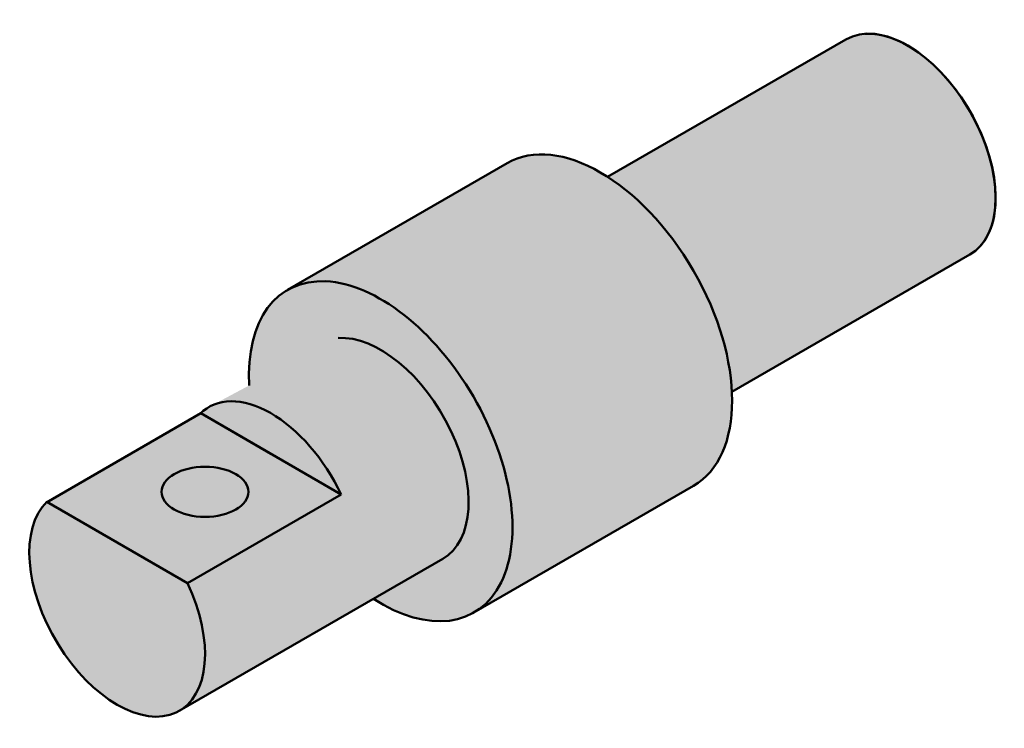
# Model space of a CAD drawing. Units: inches. Extents: x 105 to 6825, y 111 to 6061.
# Tile 1 of 2: x 105 to 299, y 111 to 250. Entities that reach past the tile are written whole.
import ezdxf

# ---------------------------------------------------------------- set-up
doc = ezdxf.new("R2010")
doc.units = ezdxf.units.IN
doc.header["$MEASUREMENT"] = 0
doc.layers.add('M-HATC', color=8, linetype='Continuous', lineweight=18)
doc.layers.add('M-OUTL', color=7, linetype='Continuous', lineweight=50)

msp = doc.modelspace()

# ---------------------------------------------------------------- hatches: boundary and pattern name
at = {"layer": 'M-HATC'}
h = msp.add_hatch(color=256, dxfattribs=at)
h.dxf.hatch_style = 1
h.set_gradient(color1=(99, 100, 102), tint=1, name='INVCYLINDER')
edge = h.paths.add_edge_path()
edge.add_ellipse((219.2829557775919, 190.3354462005651), major_axis=(18.37117307087383, -31.81980515339464), ratio=0.577350269189626, start_angle=392.8421304144117, end_angle=507.1578695855882)
edge.add_ellipse((219.2829557775919, 190.3354462005651), major_axis=(18.37117307087383, -31.81980515339464), ratio=0.577350269189626, start_angle=507.1578695855882, end_angle=540)
edge.add_line((200.9117827067181, 222.1552513539597), (157.6105125174961, 197.1552513539597))
edge.add_ellipse((175.9816855883699, 165.3354462005651), major_axis=(18.37117307087383, -31.81980515339464), ratio=0.577350269189626, start_angle=359.99999999999994, end_angle=540, ccw=False)
edge.add_line((194.3528586592437, 133.5156410471704), (237.6541288484657, 158.5156410471704))
edge.add_ellipse((219.2829557775919, 190.3354462005651), major_axis=(18.37117307087383, -31.81980515339464), ratio=0.577350269189626, start_angle=360, end_angle=392.8421304144117)
edge = h.paths.add_edge_path(flags=16)
edge.add_ellipse((197.6323206829809, 207.8354462005651), major_axis=(-8.573214099741122, 0), ratio=0.5773502691896255, start_angle=0, end_angle=360)
edge = h.paths.add_edge_path()
edge.add_ellipse((279.9047340425026, 225.3354462005651), major_axis=(12.24744871391588, -21.21320343559644), ratio=0.5773502691896262, start_angle=360, end_angle=530.6170018609903)
edge.add_ellipse((279.9047340425026, 225.3354462005651), major_axis=(12.24744871391588, -21.21320343559644), ratio=0.5773502691896262, start_angle=530.6170018609903, end_angle=540)
edge.add_line((267.6572853285871, 246.5486496361617), (220.7285710013052, 219.4543437865824))
edge.add_ellipse((219.2829557775919, 190.3354462005651), major_axis=(18.37117307087383, -31.81980515339464), ratio=0.577350269189626, start_angle=392.8421304144117, end_angle=507.1578695855882, ccw=False)
edge.add_line((245.223468429137, 177.0279369153896), (292.1521827564183, 204.1222427649685))
edge = h.paths.add_edge_path(flags=16)
edge.add_ellipse((243.8023449814453, 215.4109931062057), major_axis=(-6.123724356957945, 0), ratio=0.577350269189626, start_angle=388.5479502745485, end_angle=509.9999999999999, ccw=False)
edge.add_ellipse((243.8023449814453, 215.4109931062057), major_axis=(-6.123724356957945, 0), ratio=0.577350269189626, start_angle=329.99999999999994, end_angle=388.5479502745485, ccw=False)
edge.add_line((239.4722179625231, 217.9109931062057), (270.6491324987629, 235.9109931062057))
edge.add_ellipse((274.9792595176852, 233.4109931062057), major_axis=(-6.123724356957945, 0), ratio=0.577350269189626, start_angle=150, end_angle=329.99999999999994, ccw=False)
edge.add_line((279.3093865366074, 230.9109931062057), (248.1324720003676, 212.9109931062057))
edge = h.paths.add_edge_path()
edge.add_ellipse((175.9816855883699, 165.3354462005651), major_axis=(12.24744871391589, -21.21320343559642), ratio=0.577350269189626, start_angle=360, end_angle=530.6170018609903)
edge.add_line((167.577058087087, 187.6754647729887), (142.3182689200914, 174.1790395580179))
edge.add_ellipse((154.331050493759, 152.8354462005651), major_axis=(12.24744871391589, -21.21320343559642), ratio=0.5773502691896258, start_angle=436.10211375198594, end_angle=539.3720471364466, ccw=False)
edge.add_line((168.18745695431, 156.8354462005651), (137.8765678218547, 139.3354462005651))
edge.add_ellipse((124.0201613613036, 135.3354462005651), major_axis=(12.24744871391589, -21.21320343559642), ratio=0.577350269189626, start_angle=359.99999999999994, end_angle=436.102113751986, ccw=False)
edge.add_line((136.2676100752195, 114.1222427649686), (188.2291343022859, 144.1222427649687))
edge = h.paths.add_edge_path()
edge.add_ellipse((124.0201613613036, 135.3354462005651), major_axis=(12.24744871391589, -21.21320343559642), ratio=0.577350269189626, start_angle=360, end_angle=436.1021137519859)
edge.add_line((137.8765678218547, 139.335446200565), (124.0201613613036, 147.3354462005651))
edge.add_line((124.0201613613036, 147.3354462005651), (110.1997146436663, 155.3146848333139))
edge.add_line((110.1997146436663, 155.3146848333139), (110.0602307690168, 155.2341537807374))
edge.add_ellipse((124.0201613613036, 135.3354462005651), major_axis=(12.24744871391589, -21.21320343559642), ratio=0.577350269189626, start_angle=185.0515649198831, end_angle=360)
h = msp.add_hatch(color=256, dxfattribs=at)
h.dxf.hatch_style = 1
h.set_gradient(color1=(205, 105, 40), color2=(254, 204, 102), tint=1, name='INVCYLINDER')
edge = h.paths.add_edge_path()
edge.add_ellipse((175.9816855883699, 165.3354462005651), major_axis=(18.37117307087383, -31.81980515339464), ratio=0.577350269189626, start_angle=360, end_angle=540)
edge.add_ellipse((175.9816855883699, 165.3354462005651), major_axis=(18.37117307087383, -31.81980515339464), ratio=0.577350269189626, start_angle=540, end_angle=213.4043430439043)
edge.add_line((150.0580240784876, 178.3145911866752), (167.577058087087, 187.6754647729887))
edge.add_ellipse((175.9816855883699, 165.3354462005651), major_axis=(12.24744871391589, -21.21320343559642), ratio=0.577350269189626, start_angle=360, end_angle=530.6170018609904, ccw=False)
edge.add_line((188.2291343022859, 144.1222427649687), (174.5360703646567, 136.2165486145477))
edge.add_ellipse((175.9816855883699, 165.3354462005651), major_axis=(18.37117307087383, -31.81980515339464), ratio=0.577350269189626, start_angle=327.1578695855883, end_angle=360)
edge = h.paths.add_edge_path()
edge.add_ellipse((154.331050493759, 152.8354462005651), major_axis=(12.24744871391589, -21.21320343559642), ratio=0.5773502691896258, start_angle=436.1021137519858, end_angle=539.3720471364466)
edge.add_ellipse((154.331050493759, 152.8354462005651), major_axis=(12.24744871391589, -21.21320343559642), ratio=0.5773502691896258, start_angle=539.3720471364466, end_angle=185.0515649198831)
edge.add_line((140.4830409542333, 172.8305982359507), (168.18745695431, 156.8354462005651))
edge = h.paths.add_edge_path()
edge.add_ellipse((274.7326623839076, 228.4170778232225), major_axis=(-6.123724356957945, 0), ratio=0.577350269189626, start_angle=208.5479502745484, end_angle=329.99999999999994, ccw=False)
edge.add_line((279.1894483769248, 230.8417467774269), (279.3093865366074, 230.9109931062057))
edge.add_ellipse((274.9792595176852, 233.4109931062057), major_axis=(-6.123724356957945, 0), ratio=0.577350269189626, start_angle=149.9999999999999, end_angle=329.9999999999999)
edge.add_line((270.6491324987628, 235.9109931062056), (239.4722179625231, 217.9109931062057))
edge.add_ellipse((243.8023449814453, 215.4109931062057), major_axis=(-6.123724356957945, 0), ratio=0.577350269189626, start_angle=329.9999999999999, end_angle=388.5479502745485)
edge.add_line((239.3455589884283, 212.9863241520014), (270.4025353649857, 230.9170778232227))
h = msp.add_hatch(color=256, dxfattribs=at)
h.dxf.hatch_style = 1
h.set_gradient(color1=(205, 105, 40), color2=(254, 204, 102), tint=1, name='INVCYLINDER')
h.paths.add_polyline_path([(168.18745695431, 156.8354462005651), (140.5106037761216, 172.8146848333139), (110.1997146436663, 155.3146848333139), (124.0201613613036, 147.3354462005651), (137.8765678218547, 139.3354462005651)])
edge = h.paths.add_edge_path(flags=16)
edge.add_ellipse((141.3406694369924, 157.3354462005651), major_axis=(-8.573214099741122, 0), ratio=0.5773502691896255, start_angle=0, end_angle=360)
edge = h.paths.add_edge_path()
edge.add_ellipse((197.6323206829809, 207.8354462005651), major_axis=(-8.573214099741122, 0), ratio=0.5773502691896255, start_angle=0, end_angle=360)
edge = h.paths.add_edge_path()
edge.add_ellipse((274.7326623839076, 228.4170778232225), major_axis=(-6.123724356957945, 0), ratio=0.577350269189626, start_angle=208.5479502745484, end_angle=329.9999999999999)
edge.add_line((270.4025353649857, 230.9170778232227), (239.3455589884283, 212.9863241520014))
edge.add_ellipse((243.8023449814453, 215.4109931062057), major_axis=(-6.123724356957945, 0), ratio=0.577350269189626, start_angle=388.5479502745485, end_angle=509.9999999999999)
edge.add_line((248.1324720003674, 212.9109931062056), (279.1894483769248, 230.8417467774269))
h = msp.add_hatch(color=256, dxfattribs=at)
h.dxf.hatch_style = 1
h.set_gradient(color1=(153, 27, 30), color2=(254, 204, 102), tint=1, name='INVCYLINDER')
edge = h.paths.add_edge_path()
edge.add_ellipse((197.6323206829809, 207.8354462005651), major_axis=(-8.573214099741122, 0), ratio=0.5773502691896255, start_angle=0, end_angle=360)
edge = h.paths.add_edge_path()
edge.add_ellipse((141.3406694369924, 157.3354462005651), major_axis=(-8.573214099741122, 0), ratio=0.5773502691896255, start_angle=0, end_angle=360)

# ---------------------------------------------------------------- linework, layer by layer
at = {"layer": 'M-OUTL'}
for p, q in [((267.6572853285867, 246.5486496361615), (220.7285710013052, 219.4543437865824)), ((157.6105125174961, 197.1552513539597), (200.9117827067181, 222.1552513539597)), ((292.1521827564185, 204.1222427649686), (245.223468429137, 177.0279369153896)), ((110.0602307690168, 155.2341537807374), (140.5106037761216, 172.8146848333139)), ((154.331050493759, 164.8354462005651), (140.5106037761216, 172.8146848333139)), ((140.5106037761216, 172.8146848333139), (168.18745695431, 156.8354462005651)), ((194.3528586592438, 133.5156410471704), (237.6541288484657, 158.5156410471704)), ((124.0201613613036, 147.3354462005651), (110.1637549007526, 155.3354462005651)), ((137.8765678218547, 139.3354462005651), (168.18745695431, 156.8354462005651)), ((124.0201613613036, 147.3354462005651), (137.8765678218547, 139.3354462005651)), ((188.2291343022858, 144.1222427649686), (136.2676100752195, 114.1222427649686)), ((136.2676100752195, 114.1222427649686), (188.2291343022859, 144.1222427649687))]:
    msp.add_line(p, q, dxfattribs=at)
for centre, major_axis, ratio, start_param, end_param in [((279.9047340425026, 225.3354462005651), (12.24744871391588, -21.21320343559644), 0.5773502691896262, 6.283185307179586, 9.42477796076938), ((279.9047340425026, 225.335446200565), (12.24744871391589, -21.21320343559642), 0.577350269189626, 6.283185307179586, 9.146019019490385), ((219.2829557775919, 190.3354462005651), (18.37117307087383, -31.81980515339464), 0.577350269189626, 6.283185307179586, 9.42477796076938), ((175.9816855883699, 165.3354462005651), (18.37117307087383, -31.81980515339464), 0.577350269189626, 5.442116636611656, 10.27648764334619), ((175.9816855883699, 165.3354462005651), (12.24744871391589, -21.21320343559642), 0.577350269189626, 6.283185307179586, 9.146019019490385), ((154.331050493759, 152.8354462005651), (12.24744871391589, -21.21320343559642), 0.5773502691896257, 7.712084579370317, 9.576703848810835), ((124.0201613613036, 135.3354462005651), (12.24744871391589, -21.21320343559642), 0.577350269189626, 3.283489708193956, 7.712084579370318), ((124.0201613613036, 135.3354462005651), (12.24744871391589, -21.21320343559642), 0.577350269189626, 3.283489708193956, 7.712084579370318)]:
    msp.add_ellipse(centre, major_axis=major_axis, ratio=ratio, start_param=start_param, end_param=end_param, dxfattribs=at)
msp.add_ellipse((141.3406694369924, 157.3354462005651), major_axis=(-8.573214099741122, 0), ratio=0.5773502691896255, dxfattribs=at)

doc.saveas('drawing.dxf')
